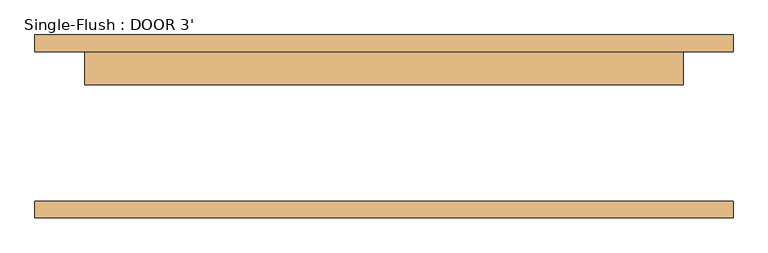
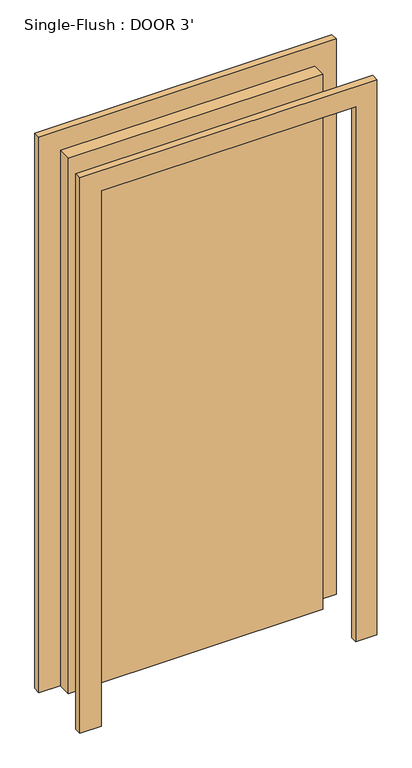
"""IFC4 building model written with IfcOpenShell, lengths in millimetres: door geometry, Single-Flush : DOOR 3'."""

from ifc_helpers import new_model, si_unit, frame, origin, origin_with_axes, place, context, project, spatial, polyline, outline, extrude, source, transform, mapped, element, save


def single_flush_door_3_89fc3733(model_context):
    return source(origin(), model_context, "Body", "SweptSolid", [
        extrude(outline(polyline([(2108.2, -533.4), (0.0, -533.4), (0.0, -457.2), (2032.0, -457.2), (2032.0, 457.2), (0.0, 457.2), (0.0, 533.4), (2108.2, 533.4), (2108.2, -533.4)])), frame((0.0, 114.3, 0.0), z_axis=(0.0, 1.0, 0.0), x_axis=(0.0, 0.0, 1.0)), (0.0, 0.0, 1.0), 25.4),
        extrude(outline(polyline([(2108.2, 533.4), (2108.2, -533.4), (0.0, -533.4), (0.0, -457.2), (2032.0, -457.2), (2032.0, 457.2), (0.0, 457.2), (0.0, 533.4), (2108.2, 533.4)])), frame((0.0, -139.7, 0.0), z_axis=(0.0, 1.0, 0.0), x_axis=(0.0, 0.0, 1.0)), (0.0, 0.0, 1.0), 25.4),
        extrude(outline(polyline([(457.2, 63.5), (-457.2, 63.5), (-457.2, 114.3), (457.2, 114.3), (457.2, 63.5)])), origin_with_axes(), (0.0, 0.0, 1.0), 2032.0),
    ])


if __name__ == "__main__":
    model = new_model("IFC4")
    model_context = context("Model", 3, world=origin())
    ifc_project = project(units=[si_unit("LENGTHUNIT", "METRE", prefix="MILLI")], contexts=[model_context])
    site = spatial("IfcSite", under=ifc_project)
    building = spatial("IfcBuilding", under=site)
    placement = place(None, origin())
    single_flush_door_3_shape = single_flush_door_3_89fc3733(model_context)
    element("IfcDoor", 1, ObjectType="Single-Flush : DOOR 3'", at=placement, inside=building, context=model_context, shape_type="MappedRepresentation", body=[
        mapped(single_flush_door_3_shape, transform((0.0, 0.0, 0.0), x_axis=(1.0, 0.0, 0.0), y_axis=(0.0, 1.0, 0.0), z_axis=(0.0, 0.0, 1.0))),
    ])
    save(model, "model.ifc")

# Revit data of these elements
# Type "Single-Flush : DOOR 3'"
#   Type Mark = "8"
#   Construction Type Id = "MDOOR"
#   Assembly Code = "C1020"
#   Analytic Construction = "Metal"
#   Thickness = 0' - 2"
#   Heat Transfer Coefficient (U) = 0.651978 BTU/(h·ft²·°F)
#   Height = 6' - 8"
#   Trim Projection Ext = 0' - 1"
#   Trim Projection Int = 0' - 1"
#   Trim Width = 0' - 3"
#   Width = 3' - 0"
#   Define Thermal Properties by = 1
#   Door Material = Door - Panel
#   Frame Material = Door - Frame
#   Visual Light Transmittance = 0
#   Solar Heat Gain Coefficient = 0
#   Function = (empty or 0)
#   Wall Closure = (empty or 0)
# Element 1 (IfcDoor, "Single-Flush : DOOR 3'")
#   Materials on its faces: "Door - Frame", "Door - Panel"
# Materials
#   "Door - Panel": class "Wood", colour RGB 210 159 95, transparency 0, Cost = 0
#   "Door - Frame": colour RGB 118 70 51, transparency 0, Cost = 0
